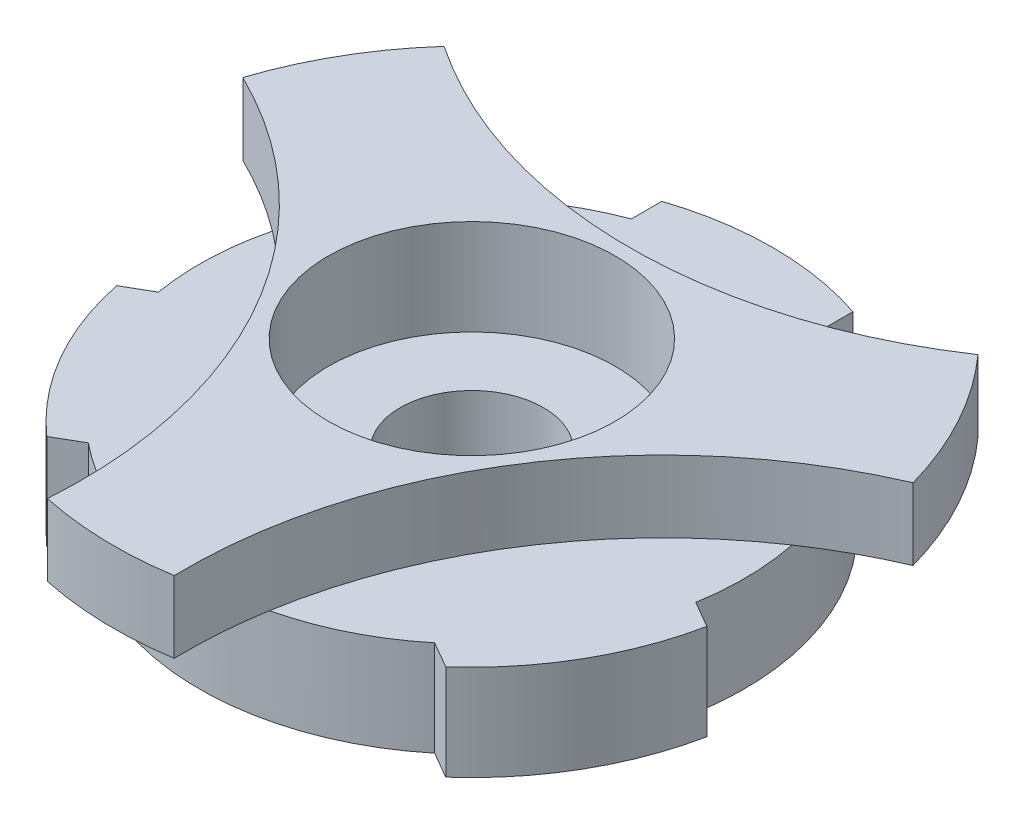
ISO-10303-21;
HEADER;
FILE_DESCRIPTION(('STEP AP214'),'2;1');
FILE_NAME('part.step','',(''),(''),'','','');
FILE_SCHEMA(('AUTOMOTIVE_DESIGN { 1 0 10303 214 1 1 1 1 }'));
ENDSEC;
DATA;
#1=APPLICATION_CONTEXT('core data for automotive mechanical design processes');
#2=APPLICATION_PROTOCOL_DEFINITION('international standard','automotive_design',2000,#1);
#3=PRODUCT_CONTEXT('',#1,'mechanical');
#4=PRODUCT('Part','Part','',(#3));
#5=PRODUCT_RELATED_PRODUCT_CATEGORY('part','',(#4));
#6=PRODUCT_DEFINITION_FORMATION('','',#4);
#7=PRODUCT_DEFINITION_CONTEXT('part definition',#1,'design');
#8=PRODUCT_DEFINITION('design','',#6,#7);
#9=PRODUCT_DEFINITION_SHAPE('','',#8);
#10=(LENGTH_UNIT() NAMED_UNIT(*) SI_UNIT(.MILLI.,.METRE.));
#11=(NAMED_UNIT(*) PLANE_ANGLE_UNIT() SI_UNIT($,.RADIAN.));
#12=(NAMED_UNIT(*) SI_UNIT($,.STERADIAN.) SOLID_ANGLE_UNIT());
#13=UNCERTAINTY_MEASURE_WITH_UNIT(LENGTH_MEASURE(1.E-05),#10,'distance_accuracy_value','');
#14=(GEOMETRIC_REPRESENTATION_CONTEXT(3) GLOBAL_UNCERTAINTY_ASSIGNED_CONTEXT((#13)) GLOBAL_UNIT_ASSIGNED_CONTEXT((#10,
#11,#12)) REPRESENTATION_CONTEXT('',''));
#15=CARTESIAN_POINT('',(0.,0.,0.));
#16=DIRECTION('',(0.,0.,1.));
#17=DIRECTION('',(1.,0.,0.));
#18=AXIS2_PLACEMENT_3D('',#15,#16,#17);
#19=CARTESIAN_POINT('',(0.,20.,0.));
#20=DIRECTION('',(0.,1.,0.));
#21=DIRECTION('',(0.,0.,1.));
#22=AXIS2_PLACEMENT_3D('',#19,#20,#21);
#23=PLANE('',#22);
#24=CARTESIAN_POINT('',(0.,20.,0.));
#25=DIRECTION('',(0.,1.,0.));
#26=DIRECTION('',(0.,0.,1.));
#27=AXIS2_PLACEMENT_3D('',#24,#25,#26);
#28=CIRCLE('',#27,57.);
#29=CARTESIAN_POINT('',(56.2249932395884,20.,9.36750421447688));
#30=VERTEX_POINT('',#29);
#31=CARTESIAN_POINT('',(55.9066338689359,20.,-11.1107285739841));
#32=VERTEX_POINT('',#31);
#33=EDGE_CURVE('E164',#30,#32,#28,.T.);
#34=ORIENTED_EDGE('',*,*,#33,.T.);
#35=CARTESIAN_POINT('',(111.776705633584,20.,71.8262057858842));
#36=DIRECTION('',(0.,1.,0.));
#37=DIRECTION('',(0.,0.,1.));
#38=AXIS2_PLACEMENT_3D('',#35,#36,#37);
#39=CIRCLE('',#38,100.);
#40=CARTESIAN_POINT('',(13.1236257711066,20.,55.4686438145007));
#41=VERTEX_POINT('',#40);
#42=EDGE_CURVE('E11',#32,#41,#39,.T.);
#43=ORIENTED_EDGE('',*,*,#42,.T.);
#44=CARTESIAN_POINT('',(0.,20.,0.));
#45=DIRECTION('',(0.,1.,0.));
#46=DIRECTION('',(0.,0.,1.));
#47=AXIS2_PLACEMENT_3D('',#44,#45,#46);
#48=CIRCLE('',#47,57.);
#49=CARTESIAN_POINT('',(36.2249932395882,20.,44.008520365854));
#50=VERTEX_POINT('',#49);
#51=EDGE_CURVE('E390',#41,#50,#48,.T.);
#52=ORIENTED_EDGE('',*,*,#51,.T.);
#53=DIRECTION('',(0.866025403784434,0.,0.500000000000007));
#54=VECTOR('',#53,1.);
#55=CARTESIAN_POINT('',(36.2249932395882,20.,44.008520365854));
#56=LINE('',#55,#54);
#57=CARTESIAN_POINT('',(41.7373172864614,20.,47.1910621381767));
#58=VERTEX_POINT('',#57);
#59=EDGE_CURVE('E391',#50,#58,#56,.T.);
#60=ORIENTED_EDGE('',*,*,#59,.T.);
#61=CARTESIAN_POINT('',(0.,20.,0.));
#62=DIRECTION('',(0.,1.,0.));
#63=DIRECTION('',(0.,0.,1.));
#64=AXIS2_PLACEMENT_3D('',#61,#62,#63);
#65=CIRCLE('',#64,63.);
#66=CARTESIAN_POINT('',(61.7373172864615,20.,12.5500459867996));
#67=VERTEX_POINT('',#66);
#68=EDGE_CURVE('E393',#58,#67,#65,.T.);
#69=ORIENTED_EDGE('',*,*,#68,.T.);
#70=DIRECTION('',(-0.866025403784435,0.,-0.500000000000007));
#71=VECTOR('',#70,1.);
#72=CARTESIAN_POINT('',(56.2249932395884,20.,9.36750421447688));
#73=LINE('',#72,#71);
#74=EDGE_CURVE('E397',#67,#30,#73,.T.);
#75=ORIENTED_EDGE('',*,*,#74,.T.);
#76=EDGE_LOOP('',(#34,#43,#52,#60,#69,#75));
#77=FACE_BOUND('',#76,.T.);
#78=ADVANCED_FACE('F43',(#77),#23,.T.);
#79=CARTESIAN_POINT('',(-36.2249932395885,20.,44.0085203658538));
#80=VERTEX_POINT('',#79);
#81=CARTESIAN_POINT('',(-15.8747051939079,20.,54.7448055527327));
#82=VERTEX_POINT('',#81);
#83=EDGE_CURVE('E387',#80,#82,#48,.T.);
#84=ORIENTED_EDGE('',*,*,#83,.T.);
#85=CARTESIAN_POINT('',(-115.18137870333,20.,66.500000000001));
#86=DIRECTION('',(0.,1.,0.));
#87=DIRECTION('',(0.,0.,1.));
#88=AXIS2_PLACEMENT_3D('',#85,#86,#87);
#89=CIRCLE('',#88,100.);
#90=CARTESIAN_POINT('',(-55.3477449308601,20.,-13.6245048008524));
#91=VERTEX_POINT('',#90);
#92=EDGE_CURVE('E55',#82,#91,#89,.T.);
#93=ORIENTED_EDGE('',*,*,#92,.T.);
#94=CARTESIAN_POINT('',(0.,20.,0.));
#95=DIRECTION('',(0.,1.,0.));
#96=DIRECTION('',(0.,0.,1.));
#97=AXIS2_PLACEMENT_3D('',#94,#95,#96);
#98=CIRCLE('',#97,57.);
#99=CARTESIAN_POINT('',(-56.2249932395883,20.,9.36750421447717));
#100=VERTEX_POINT('',#99);
#101=EDGE_CURVE('E123',#91,#100,#98,.T.);
#102=ORIENTED_EDGE('',*,*,#101,.T.);
#103=DIRECTION('',(-0.866025403784431,0.,0.500000000000014));
#104=VECTOR('',#103,1.);
#105=CARTESIAN_POINT('',(-56.2249932395883,20.,9.36750421447717));
#106=LINE('',#105,#104);
#107=CARTESIAN_POINT('',(-61.7373172864614,20.,12.5500459867999));
#108=VERTEX_POINT('',#107);
#109=EDGE_CURVE('E377',#100,#108,#106,.T.);
#110=ORIENTED_EDGE('',*,*,#109,.T.);
#111=CARTESIAN_POINT('',(0.,20.,0.));
#112=DIRECTION('',(0.,1.,0.));
#113=DIRECTION('',(0.,0.,1.));
#114=AXIS2_PLACEMENT_3D('',#111,#112,#113);
#115=CIRCLE('',#114,63.);
#116=CARTESIAN_POINT('',(-41.7373172864616,20.,47.1910621381765));
#117=VERTEX_POINT('',#116);
#118=EDGE_CURVE('E378',#108,#117,#115,.T.);
#119=ORIENTED_EDGE('',*,*,#118,.T.);
#120=DIRECTION('',(0.866025403784434,0.,-0.500000000000007));
#121=VECTOR('',#120,1.);
#122=CARTESIAN_POINT('',(-36.2249932395885,20.,44.0085203658538));
#123=LINE('',#122,#121);
#124=EDGE_CURVE('E383',#117,#80,#123,.T.);
#125=ORIENTED_EDGE('',*,*,#124,.T.);
#126=EDGE_LOOP('',(#84,#93,#102,#110,#119,#125));
#127=FACE_BOUND('',#126,.T.);
#128=ADVANCED_FACE('F413',(#127),#23,.T.);
#129=CARTESIAN_POINT('',(-20.,20.,-53.3760245803301));
#130=VERTEX_POINT('',#129);
#131=CARTESIAN_POINT('',(-39.4730397369517,20.,-41.1203007518797));
#132=VERTEX_POINT('',#131);
#133=EDGE_CURVE('E376',#130,#132,#98,.T.);
#134=ORIENTED_EDGE('',*,*,#133,.T.);
#135=CARTESIAN_POINT('',(0.,20.,-133.));
#136=DIRECTION('',(0.,1.,0.));
#137=DIRECTION('',(0.,0.,1.));
#138=AXIS2_PLACEMENT_3D('',#135,#136,#137);
#139=CIRCLE('',#138,100.);
#140=CARTESIAN_POINT('',(39.4730397369516,20.,-41.1203007518797));
#141=VERTEX_POINT('',#140);
#142=EDGE_CURVE('E234',#132,#141,#139,.T.);
#143=ORIENTED_EDGE('',*,*,#142,.T.);
#144=CARTESIAN_POINT('',(20.,20.,-53.3760245803301));
#145=VERTEX_POINT('',#144);
#146=EDGE_CURVE('E163',#141,#145,#28,.T.);
#147=ORIENTED_EDGE('',*,*,#146,.T.);
#148=DIRECTION('',(0.,0.,-1.));
#149=VECTOR('',#148,1.);
#150=CARTESIAN_POINT('',(20.,20.,-53.3760245803301));
#151=LINE('',#150,#149);
#152=CARTESIAN_POINT('',(20.,20.,-59.7411081249754));
#153=VERTEX_POINT('',#152);
#154=EDGE_CURVE('E154',#145,#153,#151,.T.);
#155=ORIENTED_EDGE('',*,*,#154,.T.);
#156=CARTESIAN_POINT('',(0.,20.,0.));
#157=DIRECTION('',(0.,1.,0.));
#158=DIRECTION('',(0.,0.,1.));
#159=AXIS2_PLACEMENT_3D('',#156,#157,#158);
#160=CIRCLE('',#159,63.);
#161=CARTESIAN_POINT('',(-20.,20.,-59.7411081249754));
#162=VERTEX_POINT('',#161);
#163=EDGE_CURVE('E159',#153,#162,#160,.T.);
#164=ORIENTED_EDGE('',*,*,#163,.T.);
#165=DIRECTION('',(0.,0.,1.));
#166=VECTOR('',#165,1.);
#167=CARTESIAN_POINT('',(-20.,20.,-53.3760245803301));
#168=LINE('',#167,#166);
#169=EDGE_CURVE('E72',#162,#130,#168,.T.);
#170=ORIENTED_EDGE('',*,*,#169,.T.);
#171=EDGE_LOOP('',(#134,#143,#147,#155,#164,#170));
#172=FACE_BOUND('',#171,.T.);
#173=ADVANCED_FACE('F155',(#172),#23,.T.);
#174=CARTESIAN_POINT('',(0.,20.,0.));
#175=DIRECTION('',(0.,-1.,0.));
#176=DIRECTION('',(0.,0.,-1.));
#177=AXIS2_PLACEMENT_3D('',#174,#175,#176);
#178=CYLINDRICAL_SURFACE('',#177,57.);
#179=CARTESIAN_POINT('',(0.,0.,0.));
#180=DIRECTION('',(0.,1.,0.));
#181=DIRECTION('',(0.,0.,1.));
#182=AXIS2_PLACEMENT_3D('',#179,#180,#181);
#183=CIRCLE('',#182,57.);
#184=CARTESIAN_POINT('',(-20.,0.,-53.3760245803301));
#185=VERTEX_POINT('',#184);
#186=CARTESIAN_POINT('',(-56.2249932395883,0.,9.36750421447717));
#187=VERTEX_POINT('',#186);
#188=EDGE_CURVE('E182',#185,#187,#183,.T.);
#189=ORIENTED_EDGE('',*,*,#188,.T.);
#190=DIRECTION('',(0.,-1.,0.));
#191=VECTOR('',#190,1.);
#192=CARTESIAN_POINT('',(-56.2249932395883,20.,9.36750421447717));
#193=LINE('',#192,#191);
#194=EDGE_CURVE('E50',#100,#187,#193,.T.);
#195=ORIENTED_EDGE('',*,*,#194,.F.);
#196=ORIENTED_EDGE('',*,*,#101,.F.);
#197=EDGE_CURVE('E366',#132,#91,#98,.T.);
#198=ORIENTED_EDGE('',*,*,#197,.F.);
#199=ORIENTED_EDGE('',*,*,#133,.F.);
#200=DIRECTION('',(0.,-1.,0.));
#201=VECTOR('',#200,1.);
#202=CARTESIAN_POINT('',(-20.,20.,-53.3760245803301));
#203=LINE('',#202,#201);
#204=EDGE_CURVE('E177',#130,#185,#203,.T.);
#205=ORIENTED_EDGE('',*,*,#204,.T.);
#206=EDGE_LOOP('',(#189,#195,#196,#198,#199,#205));
#207=FACE_BOUND('',#206,.T.);
#208=ADVANCED_FACE('F44',(#207),#178,.T.);
#209=CARTESIAN_POINT('',(-56.2249932395883,20.,9.36750421447717));
#210=DIRECTION('',(0.500000000000014,0.,0.866025403784431));
#211=DIRECTION('',(0.866025403784431,0.,-0.500000000000014));
#212=AXIS2_PLACEMENT_3D('',#209,#210,#211);
#213=PLANE('',#212);
#214=DIRECTION('',(-0.866025403784431,0.,0.500000000000014));
#215=VECTOR('',#214,1.);
#216=CARTESIAN_POINT('',(-56.2249932395883,0.,9.36750421447717));
#217=LINE('',#216,#215);
#218=CARTESIAN_POINT('',(-61.7373172864614,0.,12.5500459867999));
#219=VERTEX_POINT('',#218);
#220=EDGE_CURVE('E187',#187,#219,#217,.T.);
#221=ORIENTED_EDGE('',*,*,#220,.T.);
#222=DIRECTION('',(0.,-1.,0.));
#223=VECTOR('',#222,1.);
#224=CARTESIAN_POINT('',(-61.7373172864614,20.,12.5500459867999));
#225=LINE('',#224,#223);
#226=EDGE_CURVE('E227',#108,#219,#225,.T.);
#227=ORIENTED_EDGE('',*,*,#226,.F.);
#228=ORIENTED_EDGE('',*,*,#109,.F.);
#229=ORIENTED_EDGE('',*,*,#194,.T.);
#230=EDGE_LOOP('',(#221,#227,#228,#229));
#231=FACE_BOUND('',#230,.T.);
#232=ADVANCED_FACE('F409',(#231),#213,.F.);
#233=CARTESIAN_POINT('',(0.,20.,0.));
#234=DIRECTION('',(0.,-1.,0.));
#235=DIRECTION('',(0.,0.,-1.));
#236=AXIS2_PLACEMENT_3D('',#233,#234,#235);
#237=CYLINDRICAL_SURFACE('',#236,63.);
#238=CARTESIAN_POINT('',(0.,0.,0.));
#239=DIRECTION('',(0.,1.,0.));
#240=DIRECTION('',(0.,0.,1.));
#241=AXIS2_PLACEMENT_3D('',#238,#239,#240);
#242=CIRCLE('',#241,63.);
#243=CARTESIAN_POINT('',(-41.7373172864616,0.,47.1910621381765));
#244=VERTEX_POINT('',#243);
#245=EDGE_CURVE('E186',#219,#244,#242,.T.);
#246=ORIENTED_EDGE('',*,*,#245,.T.);
#247=DIRECTION('',(0.,-1.,0.));
#248=VECTOR('',#247,1.);
#249=CARTESIAN_POINT('',(-41.7373172864616,20.,47.1910621381765));
#250=LINE('',#249,#248);
#251=EDGE_CURVE('E223',#117,#244,#250,.T.);
#252=ORIENTED_EDGE('',*,*,#251,.F.);
#253=ORIENTED_EDGE('',*,*,#118,.F.);
#254=ORIENTED_EDGE('',*,*,#226,.T.);
#255=EDGE_LOOP('',(#246,#252,#253,#254));
#256=FACE_BOUND('',#255,.T.);
#257=ADVANCED_FACE('F412',(#256),#237,.T.);
#258=CARTESIAN_POINT('',(-36.2249932395885,20.,44.0085203658538));
#259=DIRECTION('',(-0.500000000000007,0.,-0.866025403784434));
#260=DIRECTION('',(-0.866025403784434,0.,0.500000000000008));
#261=AXIS2_PLACEMENT_3D('',#258,#259,#260);
#262=PLANE('',#261);
#263=DIRECTION('',(0.866025403784434,0.,-0.500000000000007));
#264=VECTOR('',#263,1.);
#265=CARTESIAN_POINT('',(-36.2249932395885,0.,44.0085203658538));
#266=LINE('',#265,#264);
#267=CARTESIAN_POINT('',(-36.2249932395885,0.,44.0085203658538));
#268=VERTEX_POINT('',#267);
#269=EDGE_CURVE('E191',#244,#268,#266,.T.);
#270=ORIENTED_EDGE('',*,*,#269,.T.);
#271=DIRECTION('',(0.,-1.,0.));
#272=VECTOR('',#271,1.);
#273=CARTESIAN_POINT('',(-36.2249932395885,20.,44.0085203658538));
#274=LINE('',#273,#272);
#275=EDGE_CURVE('E224',#80,#268,#274,.T.);
#276=ORIENTED_EDGE('',*,*,#275,.F.);
#277=ORIENTED_EDGE('',*,*,#124,.F.);
#278=ORIENTED_EDGE('',*,*,#251,.T.);
#279=EDGE_LOOP('',(#270,#276,#277,#278));
#280=FACE_BOUND('',#279,.T.);
#281=ADVANCED_FACE('F420',(#280),#262,.F.);
#282=CARTESIAN_POINT('',(0.,20.,0.));
#283=DIRECTION('',(0.,-1.,0.));
#284=DIRECTION('',(0.,0.,-1.));
#285=AXIS2_PLACEMENT_3D('',#282,#283,#284);
#286=CYLINDRICAL_SURFACE('',#285,57.);
#287=CARTESIAN_POINT('',(0.,0.,0.));
#288=DIRECTION('',(0.,1.,0.));
#289=DIRECTION('',(0.,0.,1.));
#290=AXIS2_PLACEMENT_3D('',#287,#288,#289);
#291=CIRCLE('',#290,57.);
#292=CARTESIAN_POINT('',(36.2249932395882,0.,44.008520365854));
#293=VERTEX_POINT('',#292);
#294=EDGE_CURVE('E192',#268,#293,#291,.T.);
#295=ORIENTED_EDGE('',*,*,#294,.T.);
#296=DIRECTION('',(0.,-1.,0.));
#297=VECTOR('',#296,1.);
#298=CARTESIAN_POINT('',(36.2249932395882,20.,44.008520365854));
#299=LINE('',#298,#297);
#300=EDGE_CURVE('E218',#50,#293,#299,.T.);
#301=ORIENTED_EDGE('',*,*,#300,.F.);
#302=ORIENTED_EDGE('',*,*,#51,.F.);
#303=EDGE_CURVE('E392',#82,#41,#48,.T.);
#304=ORIENTED_EDGE('',*,*,#303,.F.);
#305=ORIENTED_EDGE('',*,*,#83,.F.);
#306=ORIENTED_EDGE('',*,*,#275,.T.);
#307=EDGE_LOOP('',(#295,#301,#302,#304,#305,#306));
#308=FACE_BOUND('',#307,.T.);
#309=ADVANCED_FACE('F422',(#308),#286,.T.);
#310=CARTESIAN_POINT('',(36.2249932395882,20.,44.008520365854));
#311=DIRECTION('',(0.500000000000007,0.,-0.866025403784434));
#312=DIRECTION('',(-0.866025403784434,0.,-0.500000000000007));
#313=AXIS2_PLACEMENT_3D('',#310,#311,#312);
#314=PLANE('',#313);
#315=DIRECTION('',(0.866025403784434,0.,0.500000000000007));
#316=VECTOR('',#315,1.);
#317=CARTESIAN_POINT('',(36.2249932395882,0.,44.008520365854));
#318=LINE('',#317,#316);
#319=CARTESIAN_POINT('',(41.7373172864614,0.,47.1910621381767));
#320=VERTEX_POINT('',#319);
#321=EDGE_CURVE('E194',#293,#320,#318,.T.);
#322=ORIENTED_EDGE('',*,*,#321,.T.);
#323=DIRECTION('',(0.,-1.,0.));
#324=VECTOR('',#323,1.);
#325=CARTESIAN_POINT('',(41.7373172864614,20.,47.1910621381767));
#326=LINE('',#325,#324);
#327=EDGE_CURVE('E216',#58,#320,#326,.T.);
#328=ORIENTED_EDGE('',*,*,#327,.F.);
#329=ORIENTED_EDGE('',*,*,#59,.F.);
#330=ORIENTED_EDGE('',*,*,#300,.T.);
#331=EDGE_LOOP('',(#322,#328,#329,#330));
#332=FACE_BOUND('',#331,.T.);
#333=ADVANCED_FACE('F431',(#332),#314,.F.);
#334=CARTESIAN_POINT('',(0.,20.,0.));
#335=DIRECTION('',(0.,-1.,0.));
#336=DIRECTION('',(0.,0.,-1.));
#337=AXIS2_PLACEMENT_3D('',#334,#335,#336);
#338=CYLINDRICAL_SURFACE('',#337,63.);
#339=CARTESIAN_POINT('',(0.,0.,0.));
#340=DIRECTION('',(0.,1.,0.));
#341=DIRECTION('',(0.,0.,1.));
#342=AXIS2_PLACEMENT_3D('',#339,#340,#341);
#343=CIRCLE('',#342,63.);
#344=CARTESIAN_POINT('',(61.7373172864615,0.,12.5500459867996));
#345=VERTEX_POINT('',#344);
#346=EDGE_CURVE('E197',#320,#345,#343,.T.);
#347=ORIENTED_EDGE('',*,*,#346,.T.);
#348=DIRECTION('',(0.,-1.,0.));
#349=VECTOR('',#348,1.);
#350=CARTESIAN_POINT('',(61.7373172864615,20.,12.5500459867996));
#351=LINE('',#350,#349);
#352=EDGE_CURVE('E212',#67,#345,#351,.T.);
#353=ORIENTED_EDGE('',*,*,#352,.F.);
#354=ORIENTED_EDGE('',*,*,#68,.F.);
#355=ORIENTED_EDGE('',*,*,#327,.T.);
#356=EDGE_LOOP('',(#347,#353,#354,#355));
#357=FACE_BOUND('',#356,.T.);
#358=ADVANCED_FACE('F436',(#357),#338,.T.);
#359=CARTESIAN_POINT('',(56.2249932395884,20.,9.36750421447688));
#360=DIRECTION('',(-0.500000000000007,0.,0.866025403784434));
#361=DIRECTION('',(0.866025403784435,0.,0.500000000000007));
#362=AXIS2_PLACEMENT_3D('',#359,#360,#361);
#363=PLANE('',#362);
#364=DIRECTION('',(-0.866025403784435,0.,-0.500000000000007));
#365=VECTOR('',#364,1.);
#366=CARTESIAN_POINT('',(56.2249932395884,0.,9.36750421447688));
#367=LINE('',#366,#365);
#368=CARTESIAN_POINT('',(56.2249932395884,0.,9.36750421447688));
#369=VERTEX_POINT('',#368);
#370=EDGE_CURVE('E198',#345,#369,#367,.T.);
#371=ORIENTED_EDGE('',*,*,#370,.T.);
#372=DIRECTION('',(0.,-1.,0.));
#373=VECTOR('',#372,1.);
#374=CARTESIAN_POINT('',(56.2249932395884,20.,9.36750421447688));
#375=LINE('',#374,#373);
#376=EDGE_CURVE('E208',#30,#369,#375,.T.);
#377=ORIENTED_EDGE('',*,*,#376,.F.);
#378=ORIENTED_EDGE('',*,*,#74,.F.);
#379=ORIENTED_EDGE('',*,*,#352,.T.);
#380=EDGE_LOOP('',(#371,#377,#378,#379));
#381=FACE_BOUND('',#380,.T.);
#382=ADVANCED_FACE('F439',(#381),#363,.F.);
#383=CARTESIAN_POINT('',(0.,20.,0.));
#384=DIRECTION('',(0.,-1.,0.));
#385=DIRECTION('',(0.,0.,-1.));
#386=AXIS2_PLACEMENT_3D('',#383,#384,#385);
#387=CYLINDRICAL_SURFACE('',#386,57.);
#388=CARTESIAN_POINT('',(0.,0.,0.));
#389=DIRECTION('',(0.,1.,0.));
#390=DIRECTION('',(0.,0.,1.));
#391=AXIS2_PLACEMENT_3D('',#388,#389,#390);
#392=CIRCLE('',#391,57.);
#393=CARTESIAN_POINT('',(20.,0.,-53.3760245803301));
#394=VERTEX_POINT('',#393);
#395=EDGE_CURVE('E202',#369,#394,#392,.T.);
#396=ORIENTED_EDGE('',*,*,#395,.T.);
#397=DIRECTION('',(0.,-1.,0.));
#398=VECTOR('',#397,1.);
#399=CARTESIAN_POINT('',(20.,20.,-53.3760245803301));
#400=LINE('',#399,#398);
#401=EDGE_CURVE('E172',#145,#394,#400,.T.);
#402=ORIENTED_EDGE('',*,*,#401,.F.);
#403=ORIENTED_EDGE('',*,*,#146,.F.);
#404=EDGE_CURVE('E400',#32,#141,#28,.T.);
#405=ORIENTED_EDGE('',*,*,#404,.F.);
#406=ORIENTED_EDGE('',*,*,#33,.F.);
#407=ORIENTED_EDGE('',*,*,#376,.T.);
#408=EDGE_LOOP('',(#396,#402,#403,#405,#406,#407));
#409=FACE_BOUND('',#408,.T.);
#410=ADVANCED_FACE('F404',(#409),#387,.T.);
#411=CARTESIAN_POINT('',(20.,20.,-53.3760245803301));
#412=DIRECTION('',(-1.,0.,0.));
#413=DIRECTION('',(0.,0.,1.));
#414=AXIS2_PLACEMENT_3D('',#411,#412,#413);
#415=PLANE('',#414);
#416=DIRECTION('',(0.,0.,-1.));
#417=VECTOR('',#416,1.);
#418=CARTESIAN_POINT('',(20.,0.,-53.3760245803301));
#419=LINE('',#418,#417);
#420=CARTESIAN_POINT('',(20.,0.,-59.7411081249754));
#421=VERTEX_POINT('',#420);
#422=EDGE_CURVE('E171',#394,#421,#419,.T.);
#423=ORIENTED_EDGE('',*,*,#422,.T.);
#424=DIRECTION('',(0.,-1.,0.));
#425=VECTOR('',#424,1.);
#426=CARTESIAN_POINT('',(20.,20.,-59.7411081249754));
#427=LINE('',#426,#425);
#428=EDGE_CURVE('E166',#153,#421,#427,.T.);
#429=ORIENTED_EDGE('',*,*,#428,.F.);
#430=ORIENTED_EDGE('',*,*,#154,.F.);
#431=ORIENTED_EDGE('',*,*,#401,.T.);
#432=EDGE_LOOP('',(#423,#429,#430,#431));
#433=FACE_BOUND('',#432,.T.);
#434=ADVANCED_FACE('F169',(#433),#415,.F.);
#435=CARTESIAN_POINT('',(0.,20.,0.));
#436=DIRECTION('',(0.,-1.,0.));
#437=DIRECTION('',(0.,0.,-1.));
#438=AXIS2_PLACEMENT_3D('',#435,#436,#437);
#439=CYLINDRICAL_SURFACE('',#438,63.);
#440=CARTESIAN_POINT('',(0.,0.,0.));
#441=DIRECTION('',(0.,1.,0.));
#442=DIRECTION('',(0.,0.,1.));
#443=AXIS2_PLACEMENT_3D('',#440,#441,#442);
#444=CIRCLE('',#443,63.);
#445=CARTESIAN_POINT('',(-20.,0.,-59.7411081249754));
#446=VERTEX_POINT('',#445);
#447=EDGE_CURVE('E201',#421,#446,#444,.T.);
#448=ORIENTED_EDGE('',*,*,#447,.T.);
#449=DIRECTION('',(0.,-1.,0.));
#450=VECTOR('',#449,1.);
#451=CARTESIAN_POINT('',(-20.,20.,-59.7411081249754));
#452=LINE('',#451,#450);
#453=EDGE_CURVE('E174',#162,#446,#452,.T.);
#454=ORIENTED_EDGE('',*,*,#453,.F.);
#455=ORIENTED_EDGE('',*,*,#163,.F.);
#456=ORIENTED_EDGE('',*,*,#428,.T.);
#457=EDGE_LOOP('',(#448,#454,#455,#456));
#458=FACE_BOUND('',#457,.T.);
#459=ADVANCED_FACE('F180',(#458),#439,.T.);
#460=CARTESIAN_POINT('',(-20.,20.,-53.3760245803301));
#461=DIRECTION('',(1.,0.,0.));
#462=DIRECTION('',(0.,0.,-1.));
#463=AXIS2_PLACEMENT_3D('',#460,#461,#462);
#464=PLANE('',#463);
#465=DIRECTION('',(0.,0.,1.));
#466=VECTOR('',#465,1.);
#467=CARTESIAN_POINT('',(-20.,0.,-53.3760245803301));
#468=LINE('',#467,#466);
#469=EDGE_CURVE('E116',#446,#185,#468,.T.);
#470=ORIENTED_EDGE('',*,*,#469,.T.);
#471=ORIENTED_EDGE('',*,*,#204,.F.);
#472=ORIENTED_EDGE('',*,*,#169,.F.);
#473=ORIENTED_EDGE('',*,*,#453,.T.);
#474=EDGE_LOOP('',(#470,#471,#472,#473));
#475=FACE_BOUND('',#474,.T.);
#476=ADVANCED_FACE('F407',(#475),#464,.F.);
#477=CARTESIAN_POINT('',(0.,0.,0.));
#478=DIRECTION('',(0.,1.,0.));
#479=DIRECTION('',(0.,0.,1.));
#480=AXIS2_PLACEMENT_3D('',#477,#478,#479);
#481=PLANE('',#480);
#482=CARTESIAN_POINT('',(0.,0.,0.));
#483=DIRECTION('',(0.,1.,0.));
#484=DIRECTION('',(0.,0.,1.));
#485=AXIS2_PLACEMENT_3D('',#482,#483,#484);
#486=CIRCLE('',#485,15.);
#487=CARTESIAN_POINT('',(0.,0.,15.));
#488=VERTEX_POINT('',#487);
#489=EDGE_CURVE('E279',#488,#488,#486,.T.);
#490=ORIENTED_EDGE('',*,*,#489,.T.);
#491=EDGE_LOOP('',(#490));
#492=FACE_BOUND('',#491,.T.);
#493=ORIENTED_EDGE('',*,*,#188,.F.);
#494=ORIENTED_EDGE('',*,*,#469,.F.);
#495=ORIENTED_EDGE('',*,*,#447,.F.);
#496=ORIENTED_EDGE('',*,*,#422,.F.);
#497=ORIENTED_EDGE('',*,*,#395,.F.);
#498=ORIENTED_EDGE('',*,*,#370,.F.);
#499=ORIENTED_EDGE('',*,*,#346,.F.);
#500=ORIENTED_EDGE('',*,*,#321,.F.);
#501=ORIENTED_EDGE('',*,*,#294,.F.);
#502=ORIENTED_EDGE('',*,*,#269,.F.);
#503=ORIENTED_EDGE('',*,*,#245,.F.);
#504=ORIENTED_EDGE('',*,*,#220,.F.);
#505=EDGE_LOOP('',(#493,#494,#495,#496,#497,#498,#499,#500,#501,#502,#503,#504));
#506=FACE_BOUND('',#505,.T.);
#507=ADVANCED_FACE('F286',(#492,#506),#481,.F.);
#508=CARTESIAN_POINT('',(0.,20.,0.));
#509=DIRECTION('',(0.,1.,0.));
#510=DIRECTION('',(0.,0.,1.));
#511=AXIS2_PLACEMENT_3D('',#508,#509,#510);
#512=PLANE('',#511);
#513=CARTESIAN_POINT('',(-55.854579687096,20.,-50.0526315789474));
#514=VERTEX_POINT('',#513);
#515=EDGE_CURVE('E238',#514,#132,#139,.T.);
#516=ORIENTED_EDGE('',*,*,#515,.T.);
#517=ORIENTED_EDGE('',*,*,#197,.T.);
#518=CARTESIAN_POINT('',(-71.2741403171798,20.,-23.3451691372533));
#519=VERTEX_POINT('',#518);
#520=EDGE_CURVE('E241',#91,#519,#89,.T.);
#521=ORIENTED_EDGE('',*,*,#520,.T.);
#522=CARTESIAN_POINT('',(0.,20.,0.));
#523=DIRECTION('',(0.,1.,0.));
#524=DIRECTION('',(0.,0.,1.));
#525=AXIS2_PLACEMENT_3D('',#522,#523,#524);
#526=CIRCLE('',#525,75.);
#527=EDGE_CURVE('E244',#514,#519,#526,.T.);
#528=ORIENTED_EDGE('',*,*,#527,.F.);
#529=EDGE_LOOP('',(#516,#517,#521,#528));
#530=FACE_BOUND('',#529,.T.);
#531=ADVANCED_FACE('F375',(#530),#512,.F.);
#532=CARTESIAN_POINT('',(-15.419560630083,20.,73.3978007162013));
#533=VERTEX_POINT('',#532);
#534=EDGE_CURVE('E239',#533,#82,#89,.T.);
#535=ORIENTED_EDGE('',*,*,#534,.T.);
#536=ORIENTED_EDGE('',*,*,#303,.T.);
#537=CARTESIAN_POINT('',(11.8017839349531,20.,74.0656323536948));
#538=VERTEX_POINT('',#537);
#539=EDGE_CURVE('E54',#41,#538,#39,.T.);
#540=ORIENTED_EDGE('',*,*,#539,.T.);
#541=CARTESIAN_POINT('',(0.,20.,0.));
#542=DIRECTION('',(0.,1.,0.));
#543=DIRECTION('',(0.,0.,1.));
#544=AXIS2_PLACEMENT_3D('',#541,#542,#543);
#545=CIRCLE('',#544,75.);
#546=EDGE_CURVE('E273',#533,#538,#545,.T.);
#547=ORIENTED_EDGE('',*,*,#546,.F.);
#548=EDGE_LOOP('',(#535,#536,#540,#547));
#549=FACE_BOUND('',#548,.T.);
#550=ADVANCED_FACE('F549',(#549),#512,.F.);
#551=CARTESIAN_POINT('',(72.2729958770128,20.,-20.0403110495146));
#552=VERTEX_POINT('',#551);
#553=EDGE_CURVE('E53',#552,#32,#39,.T.);
#554=ORIENTED_EDGE('',*,*,#553,.T.);
#555=ORIENTED_EDGE('',*,*,#404,.T.);
#556=CARTESIAN_POINT('',(55.8545796870961,20.,-50.0526315789473));
#557=VERTEX_POINT('',#556);
#558=EDGE_CURVE('E65',#141,#557,#139,.T.);
#559=ORIENTED_EDGE('',*,*,#558,.T.);
#560=CARTESIAN_POINT('',(0.,20.,0.));
#561=DIRECTION('',(0.,1.,0.));
#562=DIRECTION('',(0.,0.,1.));
#563=AXIS2_PLACEMENT_3D('',#560,#561,#562);
#564=CIRCLE('',#563,75.);
#565=EDGE_CURVE('E246',#552,#557,#564,.T.);
#566=ORIENTED_EDGE('',*,*,#565,.F.);
#567=EDGE_LOOP('',(#554,#555,#559,#566));
#568=FACE_BOUND('',#567,.T.);
#569=ADVANCED_FACE('F405',(#568),#512,.F.);
#570=CARTESIAN_POINT('',(111.776705633584,35.,71.8262057858842));
#571=DIRECTION('',(0.,-1.,0.));
#572=DIRECTION('',(0.,0.,-1.));
#573=AXIS2_PLACEMENT_3D('',#570,#571,#572);
#574=CYLINDRICAL_SURFACE('',#573,100.);
#575=ORIENTED_EDGE('',*,*,#553,.F.);
#576=DIRECTION('',(0.,-1.,0.));
#577=VECTOR('',#576,1.);
#578=CARTESIAN_POINT('',(72.2729958770128,35.,-20.0403110495146));
#579=LINE('',#578,#577);
#580=CARTESIAN_POINT('',(72.2729958770128,35.,-20.0403110495146));
#581=VERTEX_POINT('',#580);
#582=EDGE_CURVE('E190',#581,#552,#579,.T.);
#583=ORIENTED_EDGE('',*,*,#582,.F.);
#584=CARTESIAN_POINT('',(111.776705633584,35.,71.8262057858842));
#585=DIRECTION('',(0.,1.,0.));
#586=DIRECTION('',(0.,0.,1.));
#587=AXIS2_PLACEMENT_3D('',#584,#585,#586);
#588=CIRCLE('',#587,100.);
#589=CARTESIAN_POINT('',(11.8017839349531,35.,74.0656323536948));
#590=VERTEX_POINT('',#589);
#591=EDGE_CURVE('E275',#581,#590,#588,.T.);
#592=ORIENTED_EDGE('',*,*,#591,.T.);
#593=DIRECTION('',(0.,-1.,0.));
#594=VECTOR('',#593,1.);
#595=CARTESIAN_POINT('',(11.8017839349531,35.,74.0656323536948));
#596=LINE('',#595,#594);
#597=EDGE_CURVE('E258',#590,#538,#596,.T.);
#598=ORIENTED_EDGE('',*,*,#597,.T.);
#599=ORIENTED_EDGE('',*,*,#539,.F.);
#600=ORIENTED_EDGE('',*,*,#42,.F.);
#601=EDGE_LOOP('',(#575,#583,#592,#598,#599,#600));
#602=FACE_BOUND('',#601,.T.);
#603=ADVANCED_FACE('F330',(#602),#574,.F.);
#604=CARTESIAN_POINT('',(0.,35.,0.));
#605=DIRECTION('',(0.,-1.,0.));
#606=DIRECTION('',(0.,0.,-1.));
#607=AXIS2_PLACEMENT_3D('',#604,#605,#606);
#608=CYLINDRICAL_SURFACE('',#607,75.);
#609=ORIENTED_EDGE('',*,*,#565,.T.);
#610=DIRECTION('',(0.,-1.,0.));
#611=VECTOR('',#610,1.);
#612=CARTESIAN_POINT('',(55.8545796870961,35.,-50.0526315789473));
#613=LINE('',#612,#611);
#614=CARTESIAN_POINT('',(55.8545796870961,35.,-50.0526315789473));
#615=VERTEX_POINT('',#614);
#616=EDGE_CURVE('E721',#615,#557,#613,.T.);
#617=ORIENTED_EDGE('',*,*,#616,.F.);
#618=CARTESIAN_POINT('',(0.,35.,0.));
#619=DIRECTION('',(0.,1.,0.));
#620=DIRECTION('',(0.,0.,1.));
#621=AXIS2_PLACEMENT_3D('',#618,#619,#620);
#622=CIRCLE('',#621,75.);
#623=EDGE_CURVE('E266',#581,#615,#622,.T.);
#624=ORIENTED_EDGE('',*,*,#623,.F.);
#625=ORIENTED_EDGE('',*,*,#582,.T.);
#626=EDGE_LOOP('',(#609,#617,#624,#625));
#627=FACE_BOUND('',#626,.T.);
#628=ADVANCED_FACE('F624',(#627),#608,.T.);
#629=CARTESIAN_POINT('',(0.,35.,-133.));
#630=DIRECTION('',(0.,-1.,0.));
#631=DIRECTION('',(0.,0.,-1.));
#632=AXIS2_PLACEMENT_3D('',#629,#630,#631);
#633=CYLINDRICAL_SURFACE('',#632,100.);
#634=ORIENTED_EDGE('',*,*,#515,.F.);
#635=DIRECTION('',(0.,-1.,0.));
#636=VECTOR('',#635,1.);
#637=CARTESIAN_POINT('',(-55.854579687096,35.,-50.0526315789474));
#638=LINE('',#637,#636);
#639=CARTESIAN_POINT('',(-55.854579687096,35.,-50.0526315789474));
#640=VERTEX_POINT('',#639);
#641=EDGE_CURVE('E725',#640,#514,#638,.T.);
#642=ORIENTED_EDGE('',*,*,#641,.F.);
#643=CARTESIAN_POINT('',(0.,35.,-133.));
#644=DIRECTION('',(0.,1.,0.));
#645=DIRECTION('',(0.,0.,1.));
#646=AXIS2_PLACEMENT_3D('',#643,#644,#645);
#647=CIRCLE('',#646,100.);
#648=EDGE_CURVE('E267',#640,#615,#647,.T.);
#649=ORIENTED_EDGE('',*,*,#648,.T.);
#650=ORIENTED_EDGE('',*,*,#616,.T.);
#651=ORIENTED_EDGE('',*,*,#558,.F.);
#652=ORIENTED_EDGE('',*,*,#142,.F.);
#653=EDGE_LOOP('',(#634,#642,#649,#650,#651,#652));
#654=FACE_BOUND('',#653,.T.);
#655=ADVANCED_FACE('F367',(#654),#633,.F.);
#656=CARTESIAN_POINT('',(0.,35.,0.));
#657=DIRECTION('',(0.,-1.,0.));
#658=DIRECTION('',(0.,0.,-1.));
#659=AXIS2_PLACEMENT_3D('',#656,#657,#658);
#660=CYLINDRICAL_SURFACE('',#659,75.);
#661=ORIENTED_EDGE('',*,*,#527,.T.);
#662=DIRECTION('',(0.,-1.,0.));
#663=VECTOR('',#662,1.);
#664=CARTESIAN_POINT('',(-71.2741403171798,35.,-23.3451691372533));
#665=LINE('',#664,#663);
#666=CARTESIAN_POINT('',(-71.2741403171798,35.,-23.3451691372533));
#667=VERTEX_POINT('',#666);
#668=EDGE_CURVE('E720',#667,#519,#665,.T.);
#669=ORIENTED_EDGE('',*,*,#668,.F.);
#670=CARTESIAN_POINT('',(0.,35.,0.));
#671=DIRECTION('',(0.,1.,0.));
#672=DIRECTION('',(0.,0.,1.));
#673=AXIS2_PLACEMENT_3D('',#670,#671,#672);
#674=CIRCLE('',#673,75.);
#675=EDGE_CURVE('E264',#640,#667,#674,.T.);
#676=ORIENTED_EDGE('',*,*,#675,.F.);
#677=ORIENTED_EDGE('',*,*,#641,.T.);
#678=EDGE_LOOP('',(#661,#669,#676,#677));
#679=FACE_BOUND('',#678,.T.);
#680=ADVANCED_FACE('F639',(#679),#660,.T.);
#681=CARTESIAN_POINT('',(-115.18137870333,35.,66.500000000001));
#682=DIRECTION('',(0.,-1.,0.));
#683=DIRECTION('',(0.,0.,-1.));
#684=AXIS2_PLACEMENT_3D('',#681,#682,#683);
#685=CYLINDRICAL_SURFACE('',#684,100.);
#686=ORIENTED_EDGE('',*,*,#534,.F.);
#687=DIRECTION('',(0.,-1.,0.));
#688=VECTOR('',#687,1.);
#689=CARTESIAN_POINT('',(-15.419560630083,35.,73.3978007162013));
#690=LINE('',#689,#688);
#691=CARTESIAN_POINT('',(-15.419560630083,35.,73.3978007162013));
#692=VERTEX_POINT('',#691);
#693=EDGE_CURVE('E713',#692,#533,#690,.T.);
#694=ORIENTED_EDGE('',*,*,#693,.F.);
#695=CARTESIAN_POINT('',(-115.18137870333,35.,66.500000000001));
#696=DIRECTION('',(0.,1.,0.));
#697=DIRECTION('',(0.,0.,1.));
#698=AXIS2_PLACEMENT_3D('',#695,#696,#697);
#699=CIRCLE('',#698,100.);
#700=EDGE_CURVE('E259',#692,#667,#699,.T.);
#701=ORIENTED_EDGE('',*,*,#700,.T.);
#702=ORIENTED_EDGE('',*,*,#668,.T.);
#703=ORIENTED_EDGE('',*,*,#520,.F.);
#704=ORIENTED_EDGE('',*,*,#92,.F.);
#705=EDGE_LOOP('',(#686,#694,#701,#702,#703,#704));
#706=FACE_BOUND('',#705,.T.);
#707=ADVANCED_FACE('F648',(#706),#685,.F.);
#708=CARTESIAN_POINT('',(0.,35.,0.));
#709=DIRECTION('',(0.,-1.,0.));
#710=DIRECTION('',(0.,0.,-1.));
#711=AXIS2_PLACEMENT_3D('',#708,#709,#710);
#712=CYLINDRICAL_SURFACE('',#711,75.);
#713=ORIENTED_EDGE('',*,*,#546,.T.);
#714=ORIENTED_EDGE('',*,*,#597,.F.);
#715=CARTESIAN_POINT('',(0.,35.,0.));
#716=DIRECTION('',(0.,1.,0.));
#717=DIRECTION('',(0.,0.,1.));
#718=AXIS2_PLACEMENT_3D('',#715,#716,#717);
#719=CIRCLE('',#718,75.);
#720=EDGE_CURVE('E256',#692,#590,#719,.T.);
#721=ORIENTED_EDGE('',*,*,#720,.F.);
#722=ORIENTED_EDGE('',*,*,#693,.T.);
#723=EDGE_LOOP('',(#713,#714,#721,#722));
#724=FACE_BOUND('',#723,.T.);
#725=ADVANCED_FACE('F312',(#724),#712,.T.);
#726=CARTESIAN_POINT('',(0.,35.,0.));
#727=DIRECTION('',(0.,1.,0.));
#728=DIRECTION('',(0.,0.,1.));
#729=AXIS2_PLACEMENT_3D('',#726,#727,#728);
#730=PLANE('',#729);
#731=CARTESIAN_POINT('',(0.,35.,0.));
#732=DIRECTION('',(0.,1.,0.));
#733=DIRECTION('',(0.,0.,1.));
#734=AXIS2_PLACEMENT_3D('',#731,#732,#733);
#735=CIRCLE('',#734,30.);
#736=CARTESIAN_POINT('',(0.,35.,30.));
#737=VERTEX_POINT('',#736);
#738=EDGE_CURVE('E276',#737,#737,#735,.T.);
#739=ORIENTED_EDGE('',*,*,#738,.F.);
#740=EDGE_LOOP('',(#739));
#741=FACE_BOUND('',#740,.T.);
#742=ORIENTED_EDGE('',*,*,#591,.F.);
#743=ORIENTED_EDGE('',*,*,#623,.T.);
#744=ORIENTED_EDGE('',*,*,#648,.F.);
#745=ORIENTED_EDGE('',*,*,#675,.T.);
#746=ORIENTED_EDGE('',*,*,#700,.F.);
#747=ORIENTED_EDGE('',*,*,#720,.T.);
#748=EDGE_LOOP('',(#742,#743,#744,#745,#746,#747));
#749=FACE_BOUND('',#748,.T.);
#750=ADVANCED_FACE('F310',(#741,#749),#730,.T.);
#751=CARTESIAN_POINT('',(0.,15.,0.));
#752=DIRECTION('',(0.,1.,0.));
#753=DIRECTION('',(0.,0.,1.));
#754=AXIS2_PLACEMENT_3D('',#751,#752,#753);
#755=CYLINDRICAL_SURFACE('',#754,30.);
#756=CARTESIAN_POINT('',(0.,15.,0.));
#757=DIRECTION('',(0.,1.,0.));
#758=DIRECTION('',(0.,0.,1.));
#759=AXIS2_PLACEMENT_3D('',#756,#757,#758);
#760=CIRCLE('',#759,30.);
#761=CARTESIAN_POINT('',(0.,15.,30.));
#762=VERTEX_POINT('',#761);
#763=EDGE_CURVE('E278',#762,#762,#760,.T.);
#764=ORIENTED_EDGE('',*,*,#763,.F.);
#765=EDGE_LOOP('',(#764));
#766=FACE_BOUND('',#765,.T.);
#767=ORIENTED_EDGE('',*,*,#738,.T.);
#768=EDGE_LOOP('',(#767));
#769=FACE_BOUND('',#768,.T.);
#770=ADVANCED_FACE('F301',(#766,#769),#755,.F.);
#771=CARTESIAN_POINT('',(0.,15.,0.));
#772=DIRECTION('',(0.,1.,0.));
#773=DIRECTION('',(0.,0.,1.));
#774=AXIS2_PLACEMENT_3D('',#771,#772,#773);
#775=PLANE('',#774);
#776=CARTESIAN_POINT('',(0.,15.,0.));
#777=DIRECTION('',(0.,1.,0.));
#778=DIRECTION('',(0.,0.,1.));
#779=AXIS2_PLACEMENT_3D('',#776,#777,#778);
#780=CIRCLE('',#779,15.);
#781=CARTESIAN_POINT('',(0.,15.,15.));
#782=VERTEX_POINT('',#781);
#783=EDGE_CURVE('E284',#782,#782,#780,.T.);
#784=ORIENTED_EDGE('',*,*,#783,.F.);
#785=EDGE_LOOP('',(#784));
#786=FACE_BOUND('',#785,.T.);
#787=ORIENTED_EDGE('',*,*,#763,.T.);
#788=EDGE_LOOP('',(#787));
#789=FACE_BOUND('',#788,.T.);
#790=ADVANCED_FACE('F294',(#786,#789),#775,.T.);
#791=CARTESIAN_POINT('',(0.,0.,0.));
#792=DIRECTION('',(0.,1.,0.));
#793=DIRECTION('',(0.,0.,1.));
#794=AXIS2_PLACEMENT_3D('',#791,#792,#793);
#795=CYLINDRICAL_SURFACE('',#794,15.);
#796=ORIENTED_EDGE('',*,*,#489,.F.);
#797=EDGE_LOOP('',(#796));
#798=FACE_BOUND('',#797,.T.);
#799=ORIENTED_EDGE('',*,*,#783,.T.);
#800=EDGE_LOOP('',(#799));
#801=FACE_BOUND('',#800,.T.);
#802=ADVANCED_FACE('F292',(#798,#801),#795,.F.);
#803=CLOSED_SHELL('',(#78,#128,#173,#208,#232,#257,#281,#309,#333,#358,#382,#410,#434,#459,#476,
#507,#531,#550,#569,#603,#628,#655,#680,#707,#725,#750,#770,#790,#802));
#804=MANIFOLD_SOLID_BREP('B2',#803);
#805=ADVANCED_BREP_SHAPE_REPRESENTATION('',(#18,#804),#14);
#806=SHAPE_DEFINITION_REPRESENTATION(#9,#805);
ENDSEC;
END-ISO-10303-21;
